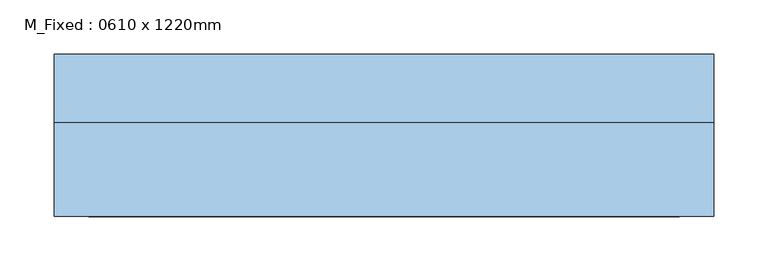
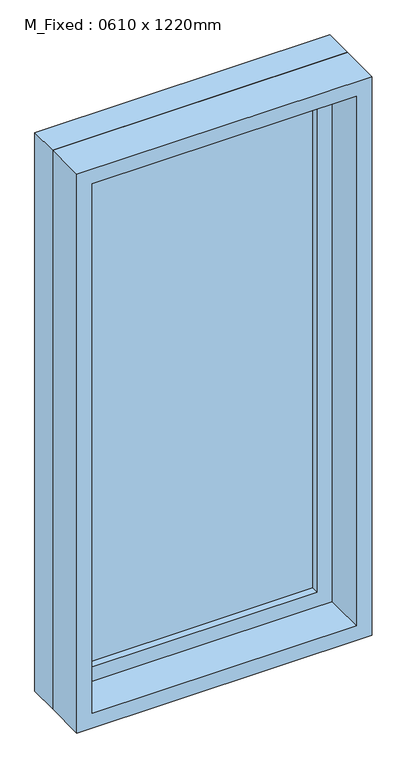
"""IFC4 building model written with IfcOpenShell, lengths in millimetres: window geometry, M_Fixed : 0610 x 1220mm."""

from ifc_helpers import new_model, si_unit, frame, origin, place, context, project, spatial, polyline, outline, extrude, source, transform, mapped, element, save


def m_fixed_0610_x_1220mm_1758882d(model_context):
    return source(origin(), model_context, "Body", "SweptSolid", [
        extrude(outline(polyline([(-242.0, 53.0), (242.0, 53.0), (242.0, 41.0), (-242.0, 41.0), (-242.0, 53.0)])), frame((0.0, 0.0, 978.0), z_axis=(0.0, 0.0, 1.0), x_axis=(1.0, 0.0, 0.0)), (0.0, 0.0, 1.0), 1094.0),
        extrude(outline(polyline([(2116.0, -286.0), (934.0, -286.0), (934.0, 286.0), (2116.0, 286.0), (2116.0, -286.0)]), holes=[polyline([(2072.0, -242.0), (2072.0, 242.0), (978.0, 242.0), (978.0, -242.0), (2072.0, -242.0)])]), frame((0.0, 25.0, 0.0), z_axis=(0.0, 1.0, 0.0), x_axis=(0.0, 0.0, 1.0)), (0.0, 0.0, 1.0), 44.0),
        extrude(outline(polyline([(2135.0, -305.0), (915.0, -305.0), (915.0, 305.0), (2135.0, 305.0), (2135.0, -305.0)]), holes=[polyline([(2116.0, -286.0), (2116.0, 286.0), (934.0, 286.0), (934.0, -286.0), (2116.0, -286.0)])]), frame((0.0, 25.0, 0.0), z_axis=(0.0, 1.0, 0.0), x_axis=(0.0, 0.0, 1.0)), (0.0, 0.0, 1.0), 63.0),
        extrude(outline(polyline([(2135.0, -305.0), (915.0, -305.0), (915.0, 305.0), (2135.0, 305.0), (2135.0, -305.0)]), holes=[polyline([(2103.0, -273.0), (2103.0, 273.0), (947.0, 273.0), (947.0, -273.0), (2103.0, -273.0)])]), frame((0.0, -62.0, 0.0), z_axis=(0.0, 1.0, 0.0), x_axis=(0.0, 0.0, 1.0)), (0.0, 0.0, 1.0), 87.0),
    ])


if __name__ == "__main__":
    model = new_model("IFC4")
    model_context = context("Model", 3, world=origin())
    ifc_project = project(units=[si_unit("LENGTHUNIT", "METRE", prefix="MILLI")], contexts=[model_context])
    site = spatial("IfcSite", under=ifc_project)
    building = spatial("IfcBuilding", under=site)
    placement = place(None, origin())
    m_fixed_0610_x_1220mm_shape = m_fixed_0610_x_1220mm_1758882d(model_context)
    element("IfcWindow", 1, ObjectType="M_Fixed : 0610 x 1220mm", at=placement, inside=building, context=model_context, shape_type="MappedRepresentation", body=[
        mapped(m_fixed_0610_x_1220mm_shape, transform((0.0, 0.0, 0.0), x_axis=(1.0, 0.0, 0.0), y_axis=(0.0, 1.0, 0.0), z_axis=(0.0, 0.0, 1.0))),
    ])
    save(model, "model.ifc")

# Revit data of these elements
# Type "M_Fixed : 0610 x 1220mm"
#   Type Mark = "13"
#   Height = 1220 mm
#   Default Sill Height = 915 mm
#   Width = 610 mm
#   Window Inset = 19 mm
#   Frame Exterior Material = Sash
#   Frame Interior Material = Sash
#   Glass Pane Material = Glass
#   Sash = Sash
#   Wall Closure = (empty or 0)
# Element 1 (IfcWindow, "M_Fixed : 0610 x 1220mm")
#   Materials on its faces: "Sash", "Glass"
# Materials
#   "Sash": class "Wood", colour RGB 136 99 55, transparency 0
#   "Glass": class "Glass", colour RGB 218 227 224, transparency 0.85, Description = "Soda Lime Glass", Cost = 0
